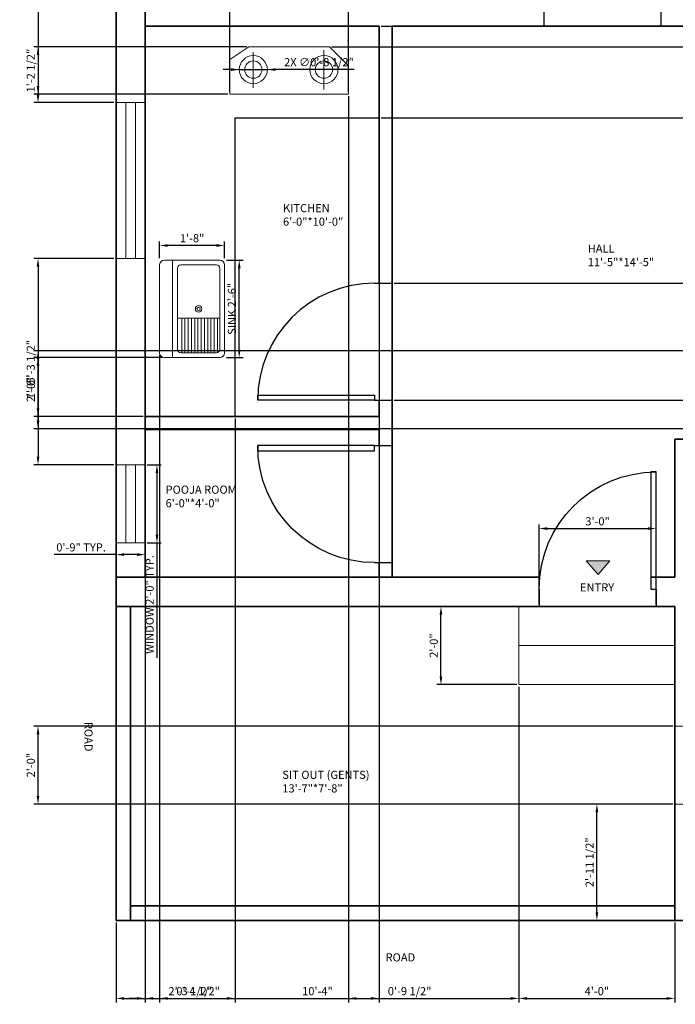
# Model space of a CAD drawing. Units: inches. Extents: x 2655 to 3059, y 1617 to 2098.
# Tile 1 of 3: x 2655 to 2857, y 1623 to 1926. Entities that reach past the tile are written whole.
import ezdxf

# ---------------------------------------------------------------- set-up
doc = ezdxf.new("R2010")
doc.units = ezdxf.units.IN
for name, color, linetype, lineweight in [('A-ANNO-DIMS', 2, 'Continuous', 18), ('A-ANNO-PATT', 7, 'Continuous', 18), ('A-ANNO-SYMB', 7, 'Continuous', 18), ('A-ANNO-TEXT', 7, 'Continuous', 18), ('A-AREA-IDEN', 7, 'Continuous', 18), ('A-DOOR', 3, 'Continuous', 25), ('A-EQPM', 8, 'Continuous', 18), ('A-FIXT-PATT', 9, 'Continuous', 13), ('A-FLOR-CASE', 8, 'Continuous', 25), ('A-FLOR-FIXT', 9, 'Continuous', 18), ('A-FLOR-STRS', 7, 'Continuous', 20), ('A-GLAZ', 4, 'Continuous', 18), ('A-WALL', 7, 'Continuous', 35)]:
    doc.layers.add(name, color=color, linetype=linetype, lineweight=lineweight)
doc.styles.get("Standard").update_dxf_attribs({"font": 'arial.ttf'})
doc.dimstyles.new('ISO-25', dxfattribs={"dimtxt": 2.5, "dimasz": 2.5, "dimexe": 1.25, "dimexo": 0.625, "dimtad": 1, "dimdec": 1, "dimlunit": 3, "dimtxsty": 'Standard', "dimcen": 2.5, "dimadec": 0, "dimazin": 0, "dimtfac": 1, "dimtdec": 1, "dimtmove": 0, "dimatfit": 3, "dimfxl": 1, "dimarcsym": 0})

# ---------------------------------------------------------------- blocks, each defined once
blk = doc.blocks.new('*U5')
for p, q in [((0, 0), (0, -6)), ((40, 0), (40, -6))]:
    blk.add_line(p, q)
blk.add_lwpolyline([(0, 0), (0, 40), (1.75, 40), (1.75, 0)], close=True)
blk.add_arc((0, 0), 40, 0, 90)
blk = doc.blocks.new('Sink-single - 30 in top')
blk.add_line((-15, -3.999996), (15, -3.999996))
for points in [[(-13.5, 0), (13.5, 0)], [(-15, -18.499996), (-15, -1.5)], [(15, -1.5), (15, -18.499996)], [(-12.5, -5.499996), (12.5, -5.499996)], [(-13.5, -17.499996), (-13.5, -6.499996)], [(13.5, -6.499996), (13.5, -17.499996)], [(13.5, -19.999996), (-13.5, -19.999996)], [(12.5, -18.499996), (-12.5, -18.499996)]]:
    blk.add_lwpolyline(points)
for radius in [1, 0.5]:
    blk.add_circle((0, -11.999996), radius)
for centre, radius, start, end in [((-13.5, -1.5), 1.5, 90, 180), ((13.5, -1.5), 1.5, 0, 90), ((-12.5, -6.499996), 1, 90, 180), ((12.5, -6.499996), 1, 0, 90), ((-12.5, -17.499996), 1, 180, 270), ((12.5, -17.499996), 1, 270, 0), ((-13.5, -18.499996), 1.5, 180, 270), ((13.5, -18.499996), 1.5, 270, 0)]:
    blk.add_arc(centre, radius, start, end)
blk = doc.blocks.new('WIN-48x9')
for p, q in [((0, 9), (48, 9)), ((0, 0), (0, 9)), ((48, 9), (48, 0)), ((0, 6), (48, 6)), ((48, 3), (0, 3)), ((48, 0), (0, 0))]:
    blk.add_line(p, q)
blk = doc.blocks.new('WIN-24x9')
for p, q in [((0, 0), (0, 24)), ((0, 24), (9, 24)), ((3, 0), (3, 24)), ((6, 24), (6, 0)), ((9, 24), (9, 0)), ((9, 0), (0, 0))]:
    blk.add_line(p, q)
blk = doc.blocks.new('*D17')
at = {"layer": 'A-ANNO-DIMS', "color": 0, "lineweight": -2, "transparency": 16777216}
for p, q in [((2694.39, 1788.85), (2698.62, 1788.85)), ((2697.37, 1786.35), (2697.37, 1767.35)), ((2694.39, 1764.85), (2698.62, 1764.85)), ((2697.37, 1764.85), (2697.37, 1729.47))]:
    blk.add_line(p, q, dxfattribs=at)
at = {"layer": 'A-ANNO-DIMS', "color": 0, "transparency": 16777216}
for points in [[(2696.95, 1786.35), (2697.79, 1786.35), (2697.37, 1788.85)], [(2696.95, 1767.35), (2697.79, 1767.35), (2697.37, 1764.85)]]:
    blk.add_solid(points, dxfattribs=at)
at = {"layer": 'Defpoints', "color": 0, "transparency": 16777216}
for p in [(2693.77, 1788.85), (2693.77, 1764.85), (2697.37, 1764.85)]:
    blk.add_point(p, dxfattribs=at)
at = {"layer": 'A-ANNO-DIMS', "color": 0, "transparency": 16777216, "insert": (2695.45, 1745.91), "char_height": 2.5, "attachment_point": 5, "rotation": 90}
blk.add_mtext('WINDOW 2\'-0" TYP.', dxfattribs=at)
blk = doc.blocks.new('*D18')
at = {"layer": 'A-ANNO-DIMS', "color": 0, "lineweight": -2, "transparency": 16777216}
for p, q in [((2684.77, 1764.23), (2684.77, 1760)), ((2693.77, 1764.23), (2693.77, 1760)), ((2684.77, 1761.25), (2665.78, 1761.25)), ((2691.27, 1761.25), (2687.27, 1761.25))]:
    blk.add_line(p, q, dxfattribs=at)
at = {"layer": 'A-ANNO-DIMS', "color": 0, "transparency": 16777216}
for points in [[(2687.27, 1761.67), (2687.27, 1760.84), (2684.77, 1761.25)], [(2691.27, 1761.67), (2691.27, 1760.84), (2693.77, 1761.25)]]:
    blk.add_solid(points, dxfattribs=at)
at = {"layer": 'Defpoints', "color": 0, "transparency": 16777216}
for p in [(2684.77, 1764.85), (2693.77, 1764.85), (2684.77, 1761.25)]:
    blk.add_point(p, dxfattribs=at)
at = {"layer": 'A-ANNO-DIMS', "color": 0, "transparency": 16777216, "insert": (2674.02, 1763.16), "char_height": 2.5, "attachment_point": 5}
blk.add_mtext('0\'-9" TYP.', dxfattribs=at)
blk = doc.blocks.new('*D21')
at = {"layer": 'A-ANNO-DIMS', "color": 0, "lineweight": -2, "transparency": 16777216}
for p, q in [((2718.82, 1851.83), (2723.94, 1851.83)), ((2722.69, 1824.33), (2722.69, 1849.33)), ((2718.82, 1821.83), (2723.94, 1821.83))]:
    blk.add_line(p, q, dxfattribs=at)
at = {"layer": 'A-ANNO-DIMS', "color": 0, "transparency": 16777216}
for points in [[(2722.28, 1849.33), (2723.11, 1849.33), (2722.69, 1851.83)], [(2722.28, 1824.33), (2723.11, 1824.33), (2722.69, 1821.83)]]:
    blk.add_solid(points, dxfattribs=at)
at = {"layer": 'Defpoints', "color": 0, "transparency": 16777216}
for p in [(2718.19, 1851.83), (2722.69, 1851.83), (2718.19, 1821.83)]:
    blk.add_point(p, dxfattribs=at)
at = {"layer": 'A-ANNO-DIMS', "color": 0, "transparency": 16777216, "insert": (2720.77, 1836.83), "char_height": 2.5, "attachment_point": 5, "rotation": 90}
blk.add_mtext('SINK 2\'-6"', dxfattribs=at)
blk = doc.blocks.new('*D22')
at = {"layer": 'A-ANNO-DIMS', "color": 0, "lineweight": -2, "transparency": 16777216}
for p, q in [((2698.19, 1852.45), (2698.19, 1857.58)), ((2715.69, 1856.33), (2700.69, 1856.33)), ((2718.19, 1852.45), (2718.19, 1857.58))]:
    blk.add_line(p, q, dxfattribs=at)
at = {"layer": 'A-ANNO-DIMS', "color": 0, "transparency": 16777216}
for points in [[(2700.69, 1856.74), (2700.69, 1855.91), (2698.19, 1856.33)], [(2715.69, 1856.74), (2715.69, 1855.91), (2718.19, 1856.33)]]:
    blk.add_solid(points, dxfattribs=at)
at = {"layer": 'Defpoints', "color": 0, "transparency": 16777216}
for p in [(2698.19, 1856.33), (2698.19, 1851.83), (2718.19, 1851.83)]:
    blk.add_point(p, dxfattribs=at)
at = {"layer": 'A-ANNO-DIMS', "color": 0, "transparency": 16777216, "insert": (2708.19, 1858.23), "char_height": 2.5, "attachment_point": 5}
blk.add_mtext('1\'-8"', dxfattribs=at)
blk = doc.blocks.new('*D24')
at = {"layer": 'A-ANNO-DIMS', "color": 0, "lineweight": -2, "transparency": 16777216}
for p, q in [((2684.14, 1975.58), (2659.52, 1975.58)), ((2660.77, 1973.08), (2660.77, 1902.78)), ((2684.15, 1900.28), (2659.52, 1900.28))]:
    blk.add_line(p, q, dxfattribs=at)
at = {"layer": 'A-ANNO-DIMS', "color": 0, "transparency": 16777216}
for points in [[(2660.35, 1973.08), (2661.19, 1973.08), (2660.77, 1975.58)], [(2660.35, 1902.78), (2661.19, 1902.78), (2660.77, 1900.28)]]:
    blk.add_solid(points, dxfattribs=at)
at = {"layer": 'Defpoints', "color": 0, "transparency": 16777216}
for p in [(2684.77, 1975.58), (2660.77, 1900.28), (2684.78, 1900.28)]:
    blk.add_point(p, dxfattribs=at)
at = {"layer": 'A-ANNO-DIMS', "color": 0, "transparency": 16777216, "insert": (2658.85, 1937.93), "char_height": 2.5, "attachment_point": 5, "rotation": 90}
blk.add_mtext('6\'-3 1/2"', dxfattribs=at)
blk = doc.blocks.new('*D25')
at = {"layer": 'A-ANNO-DIMS', "color": 0, "lineweight": -2, "transparency": 16777216}
for p, q in [((2684.15, 1852.28), (2659.52, 1852.28)), ((2660.77, 1849.78), (2660.77, 1791.35)), ((2684.14, 1788.85), (2659.52, 1788.85))]:
    blk.add_line(p, q, dxfattribs=at)
at = {"layer": 'A-ANNO-DIMS', "color": 0, "transparency": 16777216}
for points in [[(2660.35, 1849.78), (2661.19, 1849.78), (2660.77, 1852.28)], [(2660.35, 1791.35), (2661.19, 1791.35), (2660.77, 1788.85)]]:
    blk.add_solid(points, dxfattribs=at)
at = {"layer": 'Defpoints', "color": 0, "transparency": 16777216}
for p in [(2684.78, 1852.28), (2660.77, 1788.85), (2684.77, 1788.85)]:
    blk.add_point(p, dxfattribs=at)
at = {"layer": 'A-ANNO-DIMS', "color": 0, "transparency": 16777216, "insert": (2658.85, 1820.57), "char_height": 2.5, "attachment_point": 5, "rotation": 90}
blk.add_mtext('5\'-3 1/2"', dxfattribs=at)
blk = doc.blocks.new('*D30')
at = {"layer": 'A-ANNO-DIMS', "color": 0, "lineweight": -2, "transparency": 16777216}
for p, q in [((2856.14, 1684.5), (2831.52, 1684.5)), ((2832.77, 1651.27), (2832.77, 1682)), ((2856.14, 1648.77), (2831.52, 1648.77))]:
    blk.add_line(p, q, dxfattribs=at)
at = {"layer": 'A-ANNO-DIMS', "color": 0, "transparency": 16777216}
for points in [[(2832.35, 1682), (2833.19, 1682), (2832.77, 1684.5)], [(2832.35, 1651.27), (2833.19, 1651.27), (2832.77, 1648.77)]]:
    blk.add_solid(points, dxfattribs=at)
at = {"layer": 'Defpoints', "color": 0, "transparency": 16777216}
for p in [(2832.77, 1684.5), (2856.77, 1684.5), (2856.77, 1648.77)]:
    blk.add_point(p, dxfattribs=at)
at = {"layer": 'A-ANNO-DIMS', "color": 0, "transparency": 16777216, "insert": (2830.85, 1666.63), "char_height": 2.5, "attachment_point": 5, "rotation": 90}
blk.add_mtext('2\'-11 1/2"', dxfattribs=at)
blk = doc.blocks.new('*D31')
at = {"layer": 'A-ANNO-DIMS', "color": 0, "lineweight": -2, "transparency": 16777216}
for p, q in [((2856.14, 1708.5), (2659.52, 1708.5)), ((2660.77, 1687), (2660.77, 1706)), ((2856.14, 1684.5), (2659.52, 1684.5))]:
    blk.add_line(p, q, dxfattribs=at)
at = {"layer": 'A-ANNO-DIMS', "color": 0, "transparency": 16777216}
for points in [[(2660.35, 1706), (2661.19, 1706), (2660.77, 1708.5)], [(2660.35, 1687), (2661.19, 1687), (2660.77, 1684.5)]]:
    blk.add_solid(points, dxfattribs=at)
at = {"layer": 'Defpoints', "color": 0, "transparency": 16777216}
for p in [(2660.77, 1708.5), (2856.77, 1708.5), (2856.77, 1684.5)]:
    blk.add_point(p, dxfattribs=at)
at = {"layer": 'A-ANNO-DIMS', "color": 0, "transparency": 16777216, "insert": (2658.87, 1696.5), "char_height": 2.5, "attachment_point": 5, "rotation": 90}
blk.add_mtext('2\'-0"', dxfattribs=at)
blk = doc.blocks.new('*D32')
at = {"layer": 'A-ANNO-DIMS', "color": 0, "lineweight": -2, "transparency": 16777216}
for p, q in [((2808.77, 1720.64), (2808.77, 1623.52)), ((2684.77, 1648.14), (2684.77, 1623.52)), ((2687.27, 1624.77), (2806.27, 1624.77))]:
    blk.add_line(p, q, dxfattribs=at)
at = {"layer": 'A-ANNO-DIMS', "color": 0, "transparency": 16777216}
for points in [[(2687.27, 1625.18), (2687.27, 1624.35), (2684.77, 1624.77)], [(2806.27, 1625.18), (2806.27, 1624.35), (2808.77, 1624.77)]]:
    blk.add_solid(points, dxfattribs=at)
at = {"layer": 'Defpoints', "color": 0, "transparency": 16777216}
for p in [(2808.77, 1721.27), (2684.77, 1648.77), (2808.77, 1624.77)]:
    blk.add_point(p, dxfattribs=at)
at = {"layer": 'A-ANNO-DIMS', "color": 0, "transparency": 16777216, "insert": (2746.77, 1626.67), "char_height": 2.5, "attachment_point": 5}
blk.add_mtext('10\'-4"', dxfattribs=at)
blk = doc.blocks.new('*D33')
at = {"layer": 'A-ANNO-DIMS', "color": 0, "lineweight": -2, "transparency": 16777216}
for p, q in [((2808.77, 1720.64), (2808.77, 1623.52)), ((2856.77, 1648.14), (2856.77, 1623.52)), ((2811.27, 1624.77), (2854.27, 1624.77))]:
    blk.add_line(p, q, dxfattribs=at)
at = {"layer": 'A-ANNO-DIMS', "color": 0, "transparency": 16777216}
for points in [[(2811.27, 1625.18), (2811.27, 1624.35), (2808.77, 1624.77)], [(2854.27, 1625.18), (2854.27, 1624.35), (2856.77, 1624.77)]]:
    blk.add_solid(points, dxfattribs=at)
at = {"layer": 'Defpoints', "color": 0, "transparency": 16777216}
for p in [(2808.77, 1721.27), (2856.77, 1648.77), (2856.77, 1624.77)]:
    blk.add_point(p, dxfattribs=at)
at = {"layer": 'A-ANNO-DIMS', "color": 0, "transparency": 16777216, "insert": (2832.77, 1626.67), "char_height": 2.5, "attachment_point": 5}
blk.add_mtext('4\'-0"', dxfattribs=at)
blk = doc.blocks.new('*D34')
at = {"layer": 'A-ANNO-DIMS', "color": 0, "lineweight": -2, "transparency": 16777216}
for p, q in [((2814.98, 1745.89), (2814.98, 1770.52)), ((2817.48, 1769.27), (2848.48, 1769.27)), ((2850.98, 1745.89), (2850.98, 1770.52))]:
    blk.add_line(p, q, dxfattribs=at)
at = {"layer": 'A-ANNO-DIMS', "color": 0, "transparency": 16777216}
for points in [[(2817.48, 1769.68), (2817.48, 1768.85), (2814.98, 1769.27)], [(2848.48, 1769.68), (2848.48, 1768.85), (2850.98, 1769.27)]]:
    blk.add_solid(points, dxfattribs=at)
at = {"layer": 'Defpoints', "color": 0, "transparency": 16777216}
for p in [(2850.98, 1769.27), (2814.98, 1745.27), (2850.98, 1745.27)]:
    blk.add_point(p, dxfattribs=at)
at = {"layer": 'A-ANNO-DIMS', "color": 0, "transparency": 16777216, "insert": (2832.98, 1771.17), "char_height": 2.5, "attachment_point": 5}
blk.add_mtext('3\'-0"', dxfattribs=at)
blk = doc.blocks.new('*D36')
at = {"layer": 'A-ANNO-DIMS', "color": 0, "lineweight": -2, "transparency": 16777216}
for p, q in [((2808.14, 1745.27), (2783.52, 1745.27)), ((2784.77, 1723.77), (2784.77, 1742.77)), ((2808.14, 1721.27), (2783.52, 1721.27))]:
    blk.add_line(p, q, dxfattribs=at)
at = {"layer": 'A-ANNO-DIMS', "color": 0, "transparency": 16777216}
for points in [[(2784.35, 1742.77), (2785.19, 1742.77), (2784.77, 1745.27)], [(2784.35, 1723.77), (2785.19, 1723.77), (2784.77, 1721.27)]]:
    blk.add_solid(points, dxfattribs=at)
at = {"layer": 'Defpoints', "color": 0, "transparency": 16777216}
for p in [(2784.77, 1745.27), (2808.77, 1745.27), (2808.77, 1721.27)]:
    blk.add_point(p, dxfattribs=at)
at = {"layer": 'A-ANNO-DIMS', "color": 0, "transparency": 16777216, "insert": (2782.87, 1733.27), "char_height": 2.5, "attachment_point": 5, "rotation": 90}
blk.add_mtext('2\'-0"', dxfattribs=at)
blk = doc.blocks.new('*D40')
at = {"layer": 'A-ANNO-DIMS', "color": 0, "lineweight": -2, "transparency": 16777216}
for p, q in [((2949.14, 1823.93), (2659.52, 1823.93)), ((2660.77, 1802.43), (2660.77, 1821.43)), ((2949.14, 1799.93), (2659.52, 1799.93))]:
    blk.add_line(p, q, dxfattribs=at)
at = {"layer": 'A-ANNO-DIMS', "color": 0, "transparency": 16777216}
for points in [[(2660.35, 1821.43), (2661.19, 1821.43), (2660.77, 1823.93)], [(2660.35, 1802.43), (2661.19, 1802.43), (2660.77, 1799.93)]]:
    blk.add_solid(points, dxfattribs=at)
at = {"layer": 'Defpoints', "color": 0, "transparency": 16777216}
for p in [(2660.77, 1823.93), (2949.77, 1823.93), (2949.77, 1799.93)]:
    blk.add_point(p, dxfattribs=at)
at = {"layer": 'A-ANNO-DIMS', "color": 0, "transparency": 16777216, "insert": (2658.87, 1811.93), "char_height": 2.5, "attachment_point": 5, "rotation": 90}
blk.add_mtext('2\'-0"', dxfattribs=at)
blk = doc.blocks.new('*D43')
at = {"layer": 'A-ANNO-DIMS', "color": 0, "lineweight": -2, "transparency": 16777216}
for p, q in [((2693.77, 1803.14), (2693.77, 1623.52)), ((2721.45, 1803.14), (2721.45, 1623.52)), ((2696.27, 1624.77), (2718.95, 1624.77))]:
    blk.add_line(p, q, dxfattribs=at)
at = {"layer": 'A-ANNO-DIMS', "color": 0, "transparency": 16777216}
for points in [[(2696.27, 1625.18), (2696.27, 1624.35), (2693.77, 1624.77)], [(2718.95, 1625.18), (2718.95, 1624.35), (2721.45, 1624.77)]]:
    blk.add_solid(points, dxfattribs=at)
at = {"layer": 'Defpoints', "color": 0, "transparency": 16777216}
for p in [(2693.77, 1803.77), (2721.45, 1803.77), (2721.45, 1624.77)]:
    blk.add_point(p, dxfattribs=at)
at = {"layer": 'A-ANNO-DIMS', "color": 0, "transparency": 16777216, "insert": (2707.61, 1626.68), "char_height": 2.5, "attachment_point": 5}
blk.add_mtext('2\'-3 1/2"', dxfattribs=at)
blk = doc.blocks.new('*D44')
at = {"layer": 'A-ANNO-DIMS', "color": 0, "lineweight": -2, "transparency": 16777216}
for p, q in [((2766.39, 1923.77), (3058.02, 1923.77)), ((3056.77, 1898.09), (3056.77, 1921.27)), ((2766.39, 1895.59), (3058.02, 1895.59))]:
    blk.add_line(p, q, dxfattribs=at)
at = {"layer": 'A-ANNO-DIMS', "color": 0, "transparency": 16777216}
for points in [[(3056.35, 1921.27), (3057.19, 1921.27), (3056.77, 1923.77)], [(3056.35, 1898.09), (3057.19, 1898.09), (3056.77, 1895.59)]]:
    blk.add_solid(points, dxfattribs=at)
at = {"layer": 'Defpoints', "color": 0, "transparency": 16777216}
for p in [(2765.77, 1923.77), (3056.77, 1923.77), (2765.77, 1895.59)]:
    blk.add_point(p, dxfattribs=at)
at = {"layer": 'A-ANNO-DIMS', "color": 0, "transparency": 16777216, "insert": (3054.89, 1909.68), "char_height": 2.5, "attachment_point": 5, "rotation": 90}
blk.add_mtext('2\'-4"', dxfattribs=at)
blk = doc.blocks.new('*D45')
at = {"layer": 'A-ANNO-DIMS', "color": 0, "lineweight": -2, "transparency": 16777216}
for p, q in [((2770.39, 1844.73), (3058.02, 1844.73)), ((3056.77, 1811.23), (3056.77, 1842.23)), ((2770.39, 1808.73), (3058.02, 1808.73))]:
    blk.add_line(p, q, dxfattribs=at)
at = {"layer": 'A-ANNO-DIMS', "color": 0, "transparency": 16777216}
for points in [[(3056.35, 1842.23), (3057.19, 1842.23), (3056.77, 1844.73)], [(3056.35, 1811.23), (3057.19, 1811.23), (3056.77, 1808.73)]]:
    blk.add_solid(points, dxfattribs=at)
at = {"layer": 'Defpoints', "color": 0, "transparency": 16777216}
for p in [(2769.77, 1844.73), (3056.77, 1844.73), (2769.77, 1808.73)]:
    blk.add_point(p, dxfattribs=at)
at = {"layer": 'A-ANNO-DIMS', "color": 0, "transparency": 16777216, "insert": (3054.87, 1826.73), "char_height": 2.5, "attachment_point": 5, "rotation": 90}
blk.add_mtext('3\'-0"', dxfattribs=at)
blk = doc.blocks.new('*D46')
at = {"layer": 'A-ANNO-DIMS', "color": 0, "lineweight": -2, "transparency": 16777216}
for p, q in [((2719.83, 1903.48), (2719.83, 2094.02)), ((2722.33, 2092.77), (2753.77, 2092.77)), ((2756.27, 1903.48), (2756.27, 2094.02))]:
    blk.add_line(p, q, dxfattribs=at)
at = {"layer": 'A-ANNO-DIMS', "color": 0, "transparency": 16777216}
for points in [[(2722.33, 2093.18), (2722.33, 2092.35), (2719.83, 2092.77)], [(2753.77, 2093.18), (2753.77, 2092.35), (2756.27, 2092.77)]]:
    blk.add_solid(points, dxfattribs=at)
at = {"layer": 'Defpoints', "color": 0, "transparency": 16777216}
for p in [(2756.27, 2092.77), (2719.83, 1902.86), (2756.27, 1902.86)]:
    blk.add_point(p, dxfattribs=at)
at = {"layer": 'A-ANNO-DIMS', "color": 0, "transparency": 16777216, "insert": (2738.05, 2094.68), "char_height": 2.5, "attachment_point": 5}
blk.add_mtext('3\'-0 1/2"', dxfattribs=at)
blk = doc.blocks.new('*D47')
at = {"layer": 'A-ANNO-DIMS', "color": 0, "lineweight": -2, "transparency": 16777216}
for p, q in [((2725.05, 1917.37), (2659.52, 1917.37)), ((2660.77, 1914.87), (2660.77, 1905.36)), ((2719.21, 1902.86), (2659.52, 1902.86))]:
    blk.add_line(p, q, dxfattribs=at)
at = {"layer": 'A-ANNO-DIMS', "color": 0, "transparency": 16777216}
for points in [[(2660.35, 1914.87), (2661.19, 1914.87), (2660.77, 1917.37)], [(2660.35, 1905.36), (2661.19, 1905.36), (2660.77, 1902.86)]]:
    blk.add_solid(points, dxfattribs=at)
at = {"layer": 'Defpoints', "color": 0, "transparency": 16777216}
for p in [(2725.68, 1917.37), (2660.77, 1902.86), (2719.83, 1902.86)]:
    blk.add_point(p, dxfattribs=at)
at = {"layer": 'A-ANNO-DIMS', "color": 0, "transparency": 16777216, "insert": (2658.85, 1910.12), "char_height": 2.5, "attachment_point": 5, "rotation": 90}
blk.add_mtext('1\'-2 1/2"', dxfattribs=at)
blk = doc.blocks.new('*D48')
at = {"layer": 'A-ANNO-DIMS', "color": 0, "lineweight": -2, "transparency": 16777216}
for p, q in [((2699.07, 1821.83), (2659.52, 1821.83)), ((2660.77, 1806.27), (2660.77, 1819.33)), ((2693.14, 1803.77), (2659.52, 1803.77))]:
    blk.add_line(p, q, dxfattribs=at)
at = {"layer": 'A-ANNO-DIMS', "color": 0, "transparency": 16777216}
for points in [[(2660.35, 1819.33), (2661.19, 1819.33), (2660.77, 1821.83)], [(2660.35, 1806.27), (2661.19, 1806.27), (2660.77, 1803.77)]]:
    blk.add_solid(points, dxfattribs=at)
at = {"layer": 'Defpoints', "color": 0, "transparency": 16777216}
for p in [(2660.77, 1821.83), (2699.69, 1821.83), (2693.77, 1803.77)]:
    blk.add_point(p, dxfattribs=at)
at = {"layer": 'A-ANNO-DIMS', "color": 0, "transparency": 16777216, "insert": (2658.87, 1812.8), "char_height": 2.5, "attachment_point": 5, "rotation": 90}
blk.add_mtext('1\'-6"', dxfattribs=at)
blk = doc.blocks.new('*D49')
at = {"layer": 'A-ANNO-DIMS', "color": 0, "lineweight": -2, "transparency": 16777216}
for p, q in [((2756.27, 1902.23), (2756.27, 1623.52)), ((2765.77, 1894.96), (2765.77, 1623.52)), ((2758.77, 1624.77), (2763.27, 1624.77)), ((2765.77, 1624.77), (2781.99, 1624.77))]:
    blk.add_line(p, q, dxfattribs=at)
at = {"layer": 'A-ANNO-DIMS', "color": 0, "transparency": 16777216}
for points in [[(2758.77, 1625.18), (2758.77, 1624.35), (2756.27, 1624.77)], [(2763.27, 1625.18), (2763.27, 1624.35), (2765.77, 1624.77)]]:
    blk.add_solid(points, dxfattribs=at)
at = {"layer": 'Defpoints', "color": 0, "transparency": 16777216}
for p in [(2756.27, 1902.86), (2765.77, 1895.59), (2765.77, 1624.77)]:
    blk.add_point(p, dxfattribs=at)
at = {"layer": 'A-ANNO-DIMS', "color": 0, "transparency": 16777216, "insert": (2775.13, 1626.68), "char_height": 2.5, "attachment_point": 5}
blk.add_mtext('0\'-9 1/2"', dxfattribs=at)
blk = doc.blocks.new('*D50')
at = {"layer": 'A-ANNO-DIMS', "color": 0, "lineweight": -2, "transparency": 16777216}
for p, q in [((3056.77, 1923.77), (3056.77, 1939.99)), ((2766.39, 1923.77), (3058.02, 1923.77)), ((3056.77, 1919.87), (3056.77, 1921.27)), ((2751.1, 1917.37), (3058.02, 1917.37))]:
    blk.add_line(p, q, dxfattribs=at)
at = {"layer": 'A-ANNO-DIMS', "color": 0, "transparency": 16777216}
for points in [[(3056.35, 1921.27), (3057.19, 1921.27), (3056.77, 1923.77)], [(3056.35, 1919.87), (3057.19, 1919.87), (3056.77, 1917.37)]]:
    blk.add_solid(points, dxfattribs=at)
at = {"layer": 'Defpoints', "color": 0, "transparency": 16777216}
for p in [(2765.77, 1923.77), (3056.77, 1923.77), (2750.48, 1917.37)]:
    blk.add_point(p, dxfattribs=at)
at = {"layer": 'A-ANNO-DIMS', "color": 0, "transparency": 16777216, "insert": (3054.85, 1933.13), "char_height": 2.5, "attachment_point": 5, "rotation": 90}
blk.add_mtext('0\'-6 1/2"', dxfattribs=at)
blk = doc.blocks.new('*D51')
at = {"layer": 'A-ANNO-DIMS', "color": 0, "lineweight": -2, "transparency": 16777216}
for p, q in [((2698.19, 1822.7), (2698.19, 1623.52)), ((2693.77, 1803.14), (2693.77, 1623.52)), ((2691.27, 1624.77), (2688.77, 1624.77)), ((2693.77, 1624.77), (2698.19, 1624.77)), ((2700.69, 1624.77), (2716.91, 1624.77))]:
    blk.add_line(p, q, dxfattribs=at)
at = {"layer": 'A-ANNO-DIMS', "color": 0, "transparency": 16777216}
for points in [[(2691.27, 1625.18), (2691.27, 1624.35), (2693.77, 1624.77)], [(2700.69, 1625.18), (2700.69, 1624.35), (2698.19, 1624.77)]]:
    blk.add_solid(points, dxfattribs=at)
at = {"layer": 'Defpoints', "color": 0, "transparency": 16777216}
for p in [(2698.19, 1823.33), (2693.77, 1803.77), (2698.19, 1624.77)]:
    blk.add_point(p, dxfattribs=at)
at = {"layer": 'A-ANNO-DIMS', "color": 0, "transparency": 16777216, "insert": (2710.05, 1626.68), "char_height": 2.5, "attachment_point": 5}
blk.add_mtext('0\'-4 1/2"', dxfattribs=at)
blk = doc.blocks.new('*D54')
at = {"layer": 'A-ANNO-DIMS', "color": 0, "lineweight": -2, "transparency": 16777216}
for p, q in [((2720.2, 1910.41), (2717.7, 1910.41)), ((2722.7, 1910.41), (2731.35, 1910.41)), ((2758.08, 1910.41), (2733.85, 1910.41))]:
    blk.add_line(p, q, dxfattribs=at)
at = {"layer": 'A-ANNO-DIMS', "color": 0, "transparency": 16777216}
for points in [[(2720.2, 1910.83), (2720.2, 1909.99), (2722.7, 1910.41)], [(2733.85, 1910.83), (2733.85, 1909.99), (2731.35, 1910.41)]]:
    blk.add_solid(points, dxfattribs=at)
at = {"layer": 'Defpoints', "color": 0, "transparency": 16777216}
for p in [(2722.7, 1910.41), (2731.35, 1910.41)]:
    blk.add_point(p, dxfattribs=at)
at = {"layer": 'A-ANNO-DIMS', "color": 0, "transparency": 16777216, "insert": (2747.22, 1912.38), "char_height": 2.5, "attachment_point": 5, "rotation": 359.9991}
blk.add_mtext('2X ∅0\'-8 1/2"', dxfattribs=at)

msp = doc.modelspace()

# ---------------------------------------------------------------- hatches: boundary and pattern name
at = {"layer": 'A-ANNO-PATT'}
h = msp.add_hatch(color=256, dxfattribs=at)
h.dxf.hatch_style = 1
h.paths.add_polyline_path([(2836.8, 1759.32), (2829.48, 1759.32), (2833.12, 1755.13)])
at = {"layer": 'A-FIXT-PATT'}
h = msp.add_hatch(dxfattribs=at)
h.set_pattern_fill('ANSI31', color=256, scale=0.3149606, angle=45, style=0)
h.paths.add_polyline_path([(2704.58, 1823.33), (2716.48, 1823.33), (2716.48, 1833.98), (2704.58, 1833.98)])

# ---------------------------------------------------------------- linework, layer by layer
at = {"layer": 'A-ANNO-SYMB'}
for p, q in [((2829.48, 1759.32), (2836.8, 1759.32)), ((2829.48, 1759.32), (2833.12, 1755.13)), ((2833.12, 1755.13), (2836.8, 1759.32))]:
    msp.add_line(p, q, dxfattribs=at)
at = {"layer": 'A-EQPM'}
for p, q in [((2719.83, 1913.55), (2725.68, 1917.37)), ((2750.48, 1917.37), (2756.27, 1911.61)), ((2727.03, 1910.41), (2727.03, 1915.8)), ((2748.75, 1910.41), (2748.75, 1916.36)), ((2727.03, 1910.41), (2721.21, 1910.41)), ((2727.03, 1910.41), (2727.03, 1904.84)), ((2727.03, 1910.41), (2732.96, 1910.41)), ((2748.75, 1910.41), (2742.83, 1910.41)), ((2748.75, 1910.41), (2748.75, 1904.28)), ((2748.75, 1910.41), (2754.59, 1910.41))]:
    msp.add_line(p, q, dxfattribs=at)
for points in [[(2725.68, 1917.37), (2750.48, 1917.37)], [(2756.27, 1911.61), (2756.27, 1902.86), (2719.83, 1902.86), (2719.83, 1913.55)]]:
    msp.add_lwpolyline(points, dxfattribs=at)
for centre, radius in [((2727.03, 1910.41), 4.33), ((2748.75, 1910.41), 4.33), ((2727.03, 1910.41), 2.66), ((2748.75, 1910.41), 2.66)]:
    msp.add_circle(centre, radius, dxfattribs=at)
at = {"layer": 'A-FLOR-CASE'}
for p, q in [((2721.45, 1803.77), (2721.45, 1895.59)), ((2721.45, 1895.59), (2765.77, 1895.59))]:
    msp.add_line(p, q, dxfattribs=at)
at = {"layer": 'A-FLOR-FIXT'}
msp.add_line((2703.69, 1833.98), (2716.69, 1833.98), dxfattribs=at)
at = {"layer": 'A-FLOR-STRS'}
for p, q in [((2808.77, 1733.27), (2808.77, 1745.27)), ((2856.77, 1745.27), (2856.77, 1733.27)), ((2856.77, 1733.27), (2808.77, 1733.27)), ((2808.77, 1733.27), (2808.77, 1721.27)), ((2808.77, 1721.27), (2856.77, 1721.27))]:
    msp.add_line(p, q, dxfattribs=at)
at = {"layer": 'A-GLAZ'}
for p, q in [((2856.77, 1684.5), (2856.77, 1708.5)), ((2856.77, 1708.5), (2860.77, 1708.5)), ((2860.77, 1684.5), (2856.77, 1684.5))]:
    msp.add_line(p, q, dxfattribs=at)
at = {"layer": 'A-WALL'}
for p, q in [((2684.77, 1648.77), (2684.77, 2068.77)), ((2693.77, 1754.27), (2693.77, 2059.77)), ((2693.77, 1923.77), (2765.77, 1923.77)), ((2765.77, 1844.73), (2765.77, 1923.77)), ((2769.77, 1754.27), (2769.77, 1923.77)), ((2769.77, 1923.77), (3023.77, 1923.77)), ((2765.77, 1803.77), (2765.77, 1808.73)), ((2693.77, 1803.77), (2765.77, 1803.77)), ((2693.77, 1799.77), (2765.77, 1799.77)), ((2765.77, 1794.79), (2765.77, 1799.77)), ((2856.77, 1754.27), (2856.77, 1796.77)), ((2949.77, 1796.77), (2856.77, 1796.77)), ((2765.77, 1754.27), (2765.77, 1758.79)), ((2815.16, 1754.27), (2684.77, 1754.27)), ((2856.77, 1754.27), (2849.41, 1754.27)), ((2856.77, 1745.27), (2684.77, 1745.27)), ((2689.27, 1745.27), (2689.27, 1648.77)), ((2856.77, 1648.77), (2856.77, 1745.27)), ((2856.77, 1653.27), (2689.27, 1653.27)), ((3032.77, 1648.77), (2684.77, 1648.77))]:
    msp.add_line(p, q, dxfattribs=at)

# ---------------------------------------------------------------- block references
at = {"layer": 'A-DOOR', "xscale": -0.9, "yscale": 0.9, "zscale": 0.9}
for p in [(2852.47, 1929.17), (2850.98, 1750.67)]:
    msp.add_blockref('*U5', p, dxfattribs=at)
at = {"layer": 'A-DOOR', "yscale": 0.9, "zscale": 0.9, "rotation": 90}
for p, xscale in [((2764.37, 1808.73), 0.9), ((2764.37, 1794.79), -0.9)]:
    msp.add_blockref('*U5', p, dxfattribs=dict(at, xscale=xscale))
at = {"layer": 'A-FLOR-FIXT', "rotation": 90}
msp.add_blockref('Sink-single - 30 in top', (2698.19, 1836.83), dxfattribs=at)
at = {"layer": 'A-GLAZ'}
for name, p, rotation in [('WIN-48x9', (2693.78, 1852.28), 90.0000000000003), ('WIN-24x9', (2693.77, 1788.85), 180)]:
    msp.add_blockref(name, p, dxfattribs=dict(at, rotation=rotation))

# ---------------------------------------------------------------- texts
at = {"layer": 'A-ANNO-TEXT', "char_height": 2.5, "attachment_point": 1}
for s, width, insert in [('ENTRY', 24.1704, (2827.57, 1752.43)), ('ROAD', 52.9922, (2767.74, 1638.64))]:
    msp.add_mtext_dynamic_manual_height_columns(s, width=width, gutter_width=12.5, heights=[0], dxfattribs=dict(at, insert=insert))
at = {"layer": 'A-ANNO-TEXT', "insert": (2677.57, 1709.82), "char_height": 2.5, "attachment_point": 1, "rotation": 270}
msp.add_mtext_dynamic_manual_height_columns('ROAD', width=26.0033, gutter_width=12.5, heights=[0], dxfattribs=at)
at = {"layer": 'A-AREA-IDEN', "char_height": 2.5, "attachment_point": 1}
for s, width, insert in [('KITCHEN\\P6\'-0"*10\'-0"', 32.8332, (2736.16, 1869.07)), ('HALL\\P11\'-5"*14\'-5"', 84.4859, (2829.95, 1856.62)), ('POOJA ROOM\\P6\'-0"*4\'-0"', 32.3113, (2700.02, 1782.48)), ('SIT OUT (GENTS)\\P13\'-7"*7\'-8"', 70.7767, (2735.96, 1694.78))]:
    msp.add_mtext_dynamic_manual_height_columns(s, width=width, gutter_width=12.5, heights=[0], dxfattribs=dict(at, insert=insert))

# ---------------------------------------------------------------- dimensions: what is measured, and where the dimension line sits
at = {"layer": 'A-ANNO-DIMS'}
for base, p1, p2, picture, middle in [((2756.27, 2092.77), (2719.83, 1902.86), (2756.27, 1902.86), '*D46', (2738.05, 2094.68)), ((2765.77, 1624.77), (2756.27, 1902.86), (2765.77, 1895.59), '*D49', (2775.13, 1626.68)), ((2698.19, 1624.77), (2693.77, 1803.77), (2698.19, 1823.33), '*D51', (2710.05, 1626.68)), ((2721.45, 1624.77), (2693.77, 1803.77), (2721.45, 1803.77), '*D43', (2707.61, 1626.68)), ((2850.98, 1769.27), (2814.98, 1745.27), (2850.98, 1745.27), '*D34', (2832.98, 1771.17)), ((2808.77, 1624.77), (2684.77, 1648.77), (2808.77, 1721.27), '*D32', (2746.77, 1626.67)), ((2856.77, 1624.77), (2808.77, 1721.27), (2856.77, 1648.77), '*D33', (2832.77, 1626.67))]:
    dim = msp.add_linear_dim(base=base, p1=p1, p2=p2, dimstyle='ISO-25', override={"dimdec": 1, "dimlfac": 1, "dimrnd": 0, "dimzin": 1, "dimdsep": 46, "dimlunit": 4, "dimfrac": 2}, dxfattribs=at)
    dim.commit()
    dim.dimension.update_dxf_attribs({"geometry": picture, "text_midpoint": middle})
for base, p1, p2, angle, picture, middle in [((2660.77, 1900.28), (2684.77, 1975.58), (2684.78, 1900.28), 90, '*D24', (2658.85, 1937.93)), ((3056.77, 1923.77), (2750.48, 1917.37), (2765.77, 1923.77), 90, '*D50', (3054.85, 1933.13)), ((3056.77, 1923.77), (2765.77, 1895.59), (2765.77, 1923.77), 90, '*D44', (3054.89, 1909.68)), ((2660.77, 1902.86), (2725.68, 1917.37), (2719.83, 1902.86), 90, '*D47', (2658.85, 1910.12)), ((2698.19, 1856.33), (2718.19, 1851.83), (2698.19, 1851.83), 180, '*D22', (2708.19, 1858.23)), ((2660.77, 1788.85), (2684.78, 1852.28), (2684.77, 1788.85), 90, '*D25', (2658.85, 1820.57)), ((3056.77, 1844.73), (2769.77, 1808.73), (2769.77, 1844.73), 90, '*D45', (3054.87, 1826.73)), ((2660.77, 1823.93), (2949.77, 1799.93), (2949.77, 1823.93), 90, '*D40', (2658.87, 1811.93)), ((2660.77, 1821.83), (2693.77, 1803.77), (2699.69, 1821.83), 90, '*D48', (2658.87, 1812.8)), ((2784.77, 1745.27), (2808.77, 1721.27), (2808.77, 1745.27), 90, '*D36', (2782.87, 1733.27)), ((2660.77, 1708.5), (2856.77, 1684.5), (2856.77, 1708.5), 90, '*D31', (2658.87, 1696.5)), ((2832.77, 1684.5), (2856.77, 1648.77), (2856.77, 1684.5), 90, '*D30', (2830.85, 1666.63))]:
    dim = msp.add_linear_dim(base=base, p1=p1, p2=p2, angle=angle, dimstyle='ISO-25', override={"dimdec": 1, "dimlfac": 1, "dimrnd": 0, "dimzin": 1, "dimdsep": 46, "dimlunit": 4, "dimfrac": 2}, dxfattribs=at)
    dim.commit()
    dim.dimension.update_dxf_attribs({"geometry": picture, "text_midpoint": middle})
dim = msp.add_diameter_dim_2p(p1=(2722.7044, 1910.4111), p2=(2731.355, 1910.411), text='2X <>', dimstyle='ISO-25', override={"dimdec": 1, "dimlfac": 1, "dimrnd": 0, "dimzin": 1, "dimdsep": 46, "dimlunit": 4, "dimfrac": 2}, dxfattribs=at)
dim.commit()
dim.dimension.update_dxf_attribs({"geometry": '*D54', "text_midpoint": (2747.2162, 1910.4108), "dimtype": 163})
for base, p1, p2, angle, text, picture, middle in [((2722.69, 1851.83), (2718.19, 1821.83), (2718.19, 1851.83), 90, 'SINK <>', '*D21', (2720.77, 1836.83)), ((2697.37, 1764.85), (2693.77, 1788.85), (2693.77, 1764.85), 270, 'WINDOW <> TYP.', '*D17', (2695.45, 1745.91)), ((2684.77, 1761.25), (2693.77, 1764.85), (2684.77, 1764.85), 180, '<> TYP.', '*D18', (2674.02, 1763.16))]:
    dim = msp.add_linear_dim(base=base, p1=p1, p2=p2, angle=angle, text=text, dimstyle='ISO-25', override={"dimdec": 1, "dimlfac": 1, "dimrnd": 0, "dimzin": 1, "dimdsep": 46, "dimlunit": 4, "dimfrac": 2}, dxfattribs=at)
    dim.commit()
    dim.dimension.update_dxf_attribs({"geometry": picture, "text_midpoint": middle})

doc.saveas('drawing.dxf')
